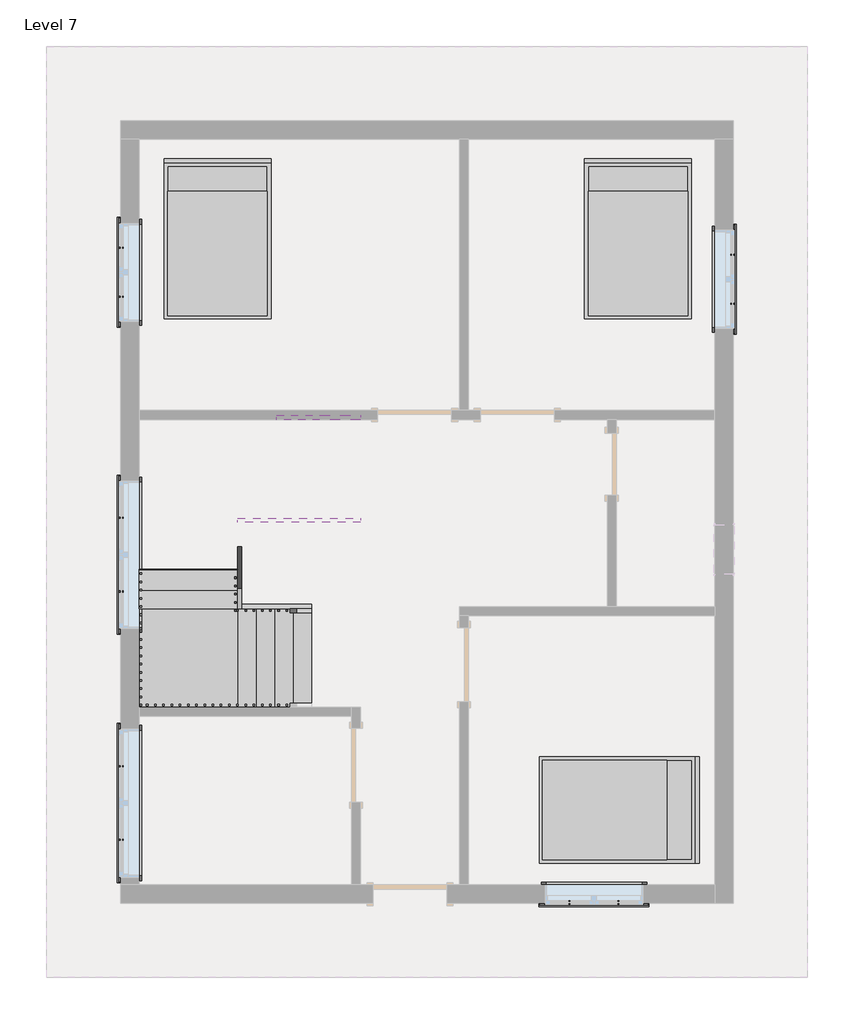
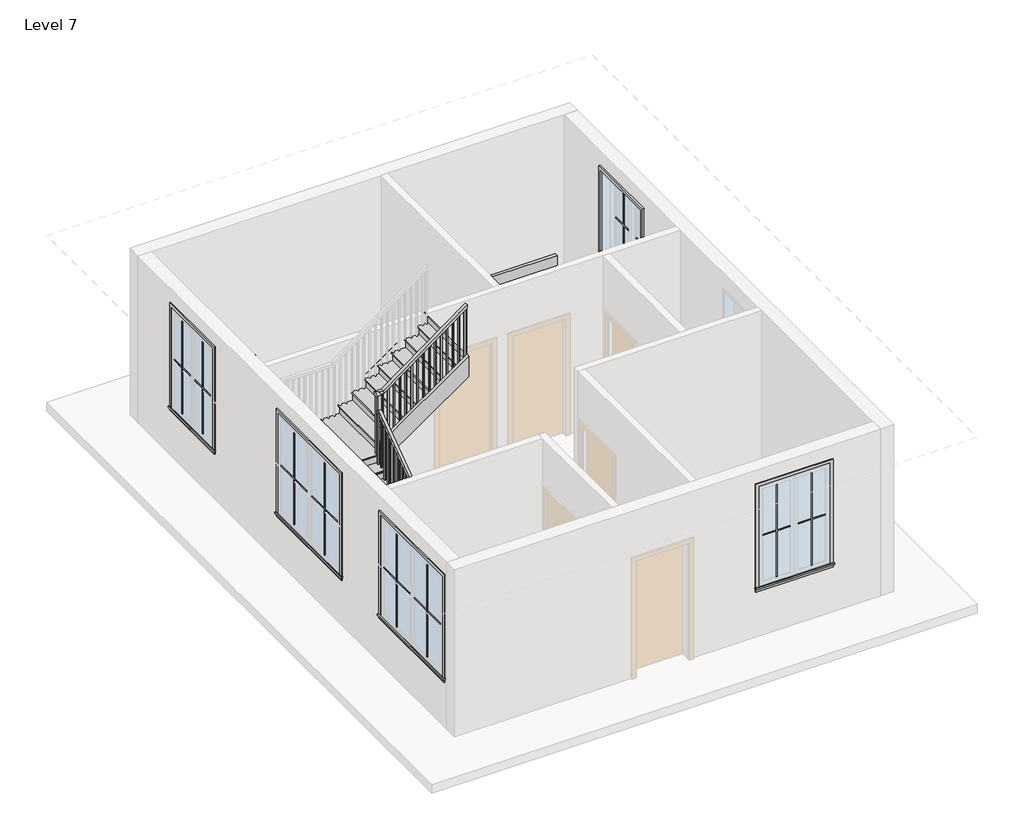
# One storey, part 3 of 3: 20 proxies, 5 members, 3 furniture elements, 1 railing, 1 stair flight.
"""IFC4 building model written with IfcOpenShell, lengths in millimetres."""

from ifc_helpers import new_model, si_unit, frame, origin, place, context, project, spatial, polyline, outline, extrude, faceted_brep, transform, mapped, element, save
from components import muntin_pattern_2x2_muntin_pattern_2x2_0a037076, muntin_pattern_2x2_muntin_pattern_2x2_e6f69628, muntin_pattern_2x2_muntin_pattern_2x2_2b4d9f72, muntin_pattern_2x2_muntin_pattern_2x2_ef995ed3, trim_window_exterior_flat_with_sill_b601e94a, trim_window_exterior_flat_with_sill_b7e4d11c, trim_window_interior_flat_picture_frame_bfefb25c, trim_window_interior_flat_picture_frame_936b8d2a, bed_17739_bed_17739_15c61121, stair_flight_f77ae209

model = new_model("IFC4")

# Units and contexts
model_context = context("Model", 3, world=origin())
ifc_project = project(units=[si_unit("LENGTHUNIT", "METRE", prefix="MILLI")], contexts=[model_context])

# Site, building, storey
site = spatial("IfcSite", under=ifc_project)
building = spatial("IfcBuilding", under=site)
storey = spatial("IfcBuildingStorey", under=building, Name="Level 7", Elevation=19050.0)

# Proxies
placement = place(None, origin())
muntin_pattern_2x2_muntin_pattern_2x2_shape = muntin_pattern_2x2_muntin_pattern_2x2_0a037076(model_context)
element("IfcBuildingElementProxy", 1, Name="Muntin Pattern_2x2 : Muntin Pattern_2x2", ObjectType="Muntin Pattern_2x2 : Muntin Pattern_2x2", at=placement, inside=storey, context=model_context, shape_type="MappedRepresentation", body=[
    mapped(muntin_pattern_2x2_muntin_pattern_2x2_shape, transform((-5035.7855391, -4380.9248761, 20034.25), x_axis=(0.0, 1.0, 0.0), y_axis=(-1.0, 0.0, 0.0), z_axis=(0.0, 0.0, 1.0))),
])
element("IfcBuildingElementProxy", 2, Name="Muntin Pattern_2x2 : Muntin Pattern_2x2", ObjectType="Muntin Pattern_2x2 : Muntin Pattern_2x2", at=placement, inside=storey, context=model_context, shape_type="MappedRepresentation", body=[
    mapped(muntin_pattern_2x2_muntin_pattern_2x2_shape, transform((-5035.7855391, -1310.6998761, 20034.25), x_axis=(0.0, 1.0, 0.0), y_axis=(-1.0, 0.0, 0.0), z_axis=(0.0, 0.0, 1.0))),
])
muntin_pattern_2x2_muntin_pattern_2x2_2_shape = muntin_pattern_2x2_muntin_pattern_2x2_e6f69628(model_context)
element("IfcBuildingElementProxy", 3, Name="Muntin Pattern_2x2 : Muntin Pattern_2x2", ObjectType="Muntin Pattern_2x2 : Muntin Pattern_2x2", at=placement, inside=storey, context=model_context, shape_type="MappedRepresentation", body=[
    mapped(muntin_pattern_2x2_muntin_pattern_2x2_2_shape, transform((-5035.7855391, -3469.6998761, 20034.25), x_axis=(0.0, -1.0, 0.0), y_axis=(1.0, 0.0, 0.0), z_axis=(0.0, 0.0, 1.0))),
])
element("IfcBuildingElementProxy", 4, Name="Muntin Pattern_2x2 : Muntin Pattern_2x2", ObjectType="Muntin Pattern_2x2 : Muntin Pattern_2x2", at=placement, inside=storey, context=model_context, shape_type="MappedRepresentation", body=[
    mapped(muntin_pattern_2x2_muntin_pattern_2x2_2_shape, transform((-5035.7855391, -399.4748761, 20034.25), x_axis=(0.0, -1.0, 0.0), y_axis=(1.0, 0.0, 0.0), z_axis=(0.0, 0.0, 1.0))),
])
muntin_pattern_2x2_muntin_pattern_2x2_3_shape = muntin_pattern_2x2_muntin_pattern_2x2_2b4d9f72(model_context)
element("IfcBuildingElementProxy", 5, Name="Muntin Pattern_2x2 : Muntin Pattern_2x2", ObjectType="Muntin Pattern_2x2 : Muntin Pattern_2x2", at=placement, inside=storey, context=model_context, shape_type="MappedRepresentation", body=[
    mapped(muntin_pattern_2x2_muntin_pattern_2x2_3_shape, transform((1115.7769609, -5157.2123761, 20034.25), x_axis=(-1.0, 0.0, 0.0), y_axis=(0.0, -1.0, 0.0), z_axis=(0.0, 0.0, 1.0))),
])
element("IfcBuildingElementProxy", 6, Name="Muntin Pattern_2x2 : Muntin Pattern_2x2", ObjectType="Muntin Pattern_2x2 : Muntin Pattern_2x2", at=placement, inside=storey, context=model_context, shape_type="MappedRepresentation", body=[
    mapped(muntin_pattern_2x2_muntin_pattern_2x2_3_shape, transform((2527.0644609, 2851.7251239, 20034.25), x_axis=(0.0, -1.0, 0.0), y_axis=(1.0, 0.0, 0.0), z_axis=(0.0, 0.0, 1.0))),
])
element("IfcBuildingElementProxy", 7, Name="Muntin Pattern_2x2 : Muntin Pattern_2x2", ObjectType="Muntin Pattern_2x2 : Muntin Pattern_2x2", at=placement, inside=storey, context=model_context, shape_type="MappedRepresentation", body=[
    mapped(muntin_pattern_2x2_muntin_pattern_2x2_3_shape, transform((-5035.7855391, 2331.0251239, 20034.25), x_axis=(0.0, 1.0, 0.0), y_axis=(-1.0, 0.0, 0.0), z_axis=(0.0, 0.0, 1.0))),
])
muntin_pattern_2x2_muntin_pattern_2x2_4_shape = muntin_pattern_2x2_muntin_pattern_2x2_ef995ed3(model_context)
element("IfcBuildingElementProxy", 8, Name="Muntin Pattern_2x2 : Muntin Pattern_2x2", ObjectType="Muntin Pattern_2x2 : Muntin Pattern_2x2", at=placement, inside=storey, context=model_context, shape_type="MappedRepresentation", body=[
    mapped(muntin_pattern_2x2_muntin_pattern_2x2_4_shape, transform((509.3519609, -5157.2123761, 20034.25), x_axis=(1.0, 0.0, 0.0), y_axis=(0.0, 1.0, 0.0), z_axis=(0.0, 0.0, 1.0))),
])
element("IfcBuildingElementProxy", 9, Name="Muntin Pattern_2x2 : Muntin Pattern_2x2", ObjectType="Muntin Pattern_2x2 : Muntin Pattern_2x2", at=placement, inside=storey, context=model_context, shape_type="MappedRepresentation", body=[
    mapped(muntin_pattern_2x2_muntin_pattern_2x2_4_shape, transform((2527.0644609, 2245.3001239, 20034.25), x_axis=(0.0, 1.0, 0.0), y_axis=(-1.0, 0.0, 0.0), z_axis=(0.0, 0.0, 1.0))),
])
element("IfcBuildingElementProxy", 10, Name="Muntin Pattern_2x2 : Muntin Pattern_2x2", ObjectType="Muntin Pattern_2x2 : Muntin Pattern_2x2", at=placement, inside=storey, context=model_context, shape_type="MappedRepresentation", body=[
    mapped(muntin_pattern_2x2_muntin_pattern_2x2_4_shape, transform((-5035.7855391, 2937.4501239, 20034.25), x_axis=(0.0, -1.0, 0.0), y_axis=(1.0, 0.0, 0.0), z_axis=(0.0, 0.0, 1.0))),
])
trim_window_exterior_flat_with_sill_shape = trim_window_exterior_flat_with_sill_b601e94a(model_context)
element("IfcBuildingElementProxy", 11, Name="Trim-Window-Exterior-Flat : with Sill", ObjectType="Trim-Window-Exterior-Flat : with Sill", at=placement, inside=storey, context=model_context, shape_type="MappedRepresentation", body=[
    mapped(trim_window_exterior_flat_with_sill_shape, transform((-5045.3105391, -3925.3123761, 21793.2), x_axis=(0.0, -1.0, 0.0), y_axis=(0.0, 0.0, 1.0), z_axis=(-1.0, 0.0, 0.0))),
])
element("IfcBuildingElementProxy", 12, Name="Trim-Window-Exterior-Flat : with Sill", ObjectType="Trim-Window-Exterior-Flat : with Sill", at=placement, inside=storey, context=model_context, shape_type="MappedRepresentation", body=[
    mapped(trim_window_exterior_flat_with_sill_shape, transform((-5045.3105391, -855.0873761, 21793.2), x_axis=(0.0, -1.0, 0.0), y_axis=(0.0, 0.0, 1.0), z_axis=(-1.0, 0.0, 0.0))),
])
trim_window_exterior_flat_with_sill_2_shape = trim_window_exterior_flat_with_sill_b7e4d11c(model_context)
element("IfcBuildingElementProxy", 13, Name="Trim-Window-Exterior-Flat : with Sill", ObjectType="Trim-Window-Exterior-Flat : with Sill", at=placement, inside=storey, context=model_context, shape_type="MappedRepresentation", body=[
    mapped(trim_window_exterior_flat_with_sill_2_shape, transform((812.5644609, -5166.7373761, 21793.2), x_axis=(1.0, 0.0, 0.0), y_axis=(0.0, 0.0, 1.0), z_axis=(0.0, -1.0, 0.0))),
])
element("IfcBuildingElementProxy", 14, Name="Trim-Window-Exterior-Flat : with Sill", ObjectType="Trim-Window-Exterior-Flat : with Sill", at=placement, inside=storey, context=model_context, shape_type="MappedRepresentation", body=[
    mapped(trim_window_exterior_flat_with_sill_2_shape, transform((2536.5894609, 2548.5126239, 21793.2), x_axis=(0.0, 1.0, 0.0), y_axis=(0.0, 0.0, 1.0), z_axis=(1.0, 0.0, 0.0))),
])
element("IfcBuildingElementProxy", 15, Name="Trim-Window-Exterior-Flat : with Sill", ObjectType="Trim-Window-Exterior-Flat : with Sill", at=placement, inside=storey, context=model_context, shape_type="MappedRepresentation", body=[
    mapped(trim_window_exterior_flat_with_sill_2_shape, transform((-5045.3105391, 2634.2376239, 21793.2), x_axis=(0.0, -1.0, 0.0), y_axis=(0.0, 0.0, 1.0), z_axis=(-1.0, 0.0, 0.0))),
])
trim_window_interior_flat_picture_frame_shape = trim_window_interior_flat_picture_frame_bfefb25c(model_context)
element("IfcBuildingElementProxy", 16, Name="Trim-Window-Interior-Flat : Picture Frame", ObjectType="Trim-Window-Interior-Flat : Picture Frame", at=placement, inside=storey, context=model_context, shape_type="MappedRepresentation", body=[
    mapped(trim_window_interior_flat_picture_frame_shape, transform((-4816.7105391, -3925.3123761, 21793.2), x_axis=(0.0, 1.0, 0.0), y_axis=(0.0, 0.0, 1.0), z_axis=(1.0, 0.0, 0.0))),
])
element("IfcBuildingElementProxy", 17, Name="Trim-Window-Interior-Flat : Picture Frame", ObjectType="Trim-Window-Interior-Flat : Picture Frame", at=placement, inside=storey, context=model_context, shape_type="MappedRepresentation", body=[
    mapped(trim_window_interior_flat_picture_frame_shape, transform((-4816.7105391, -855.0873761, 21793.2), x_axis=(0.0, 1.0, 0.0), y_axis=(0.0, 0.0, 1.0), z_axis=(1.0, 0.0, 0.0))),
])
trim_window_interior_flat_picture_frame_2_shape = trim_window_interior_flat_picture_frame_936b8d2a(model_context)
element("IfcBuildingElementProxy", 18, Name="Trim-Window-Interior-Flat : Picture Frame", ObjectType="Trim-Window-Interior-Flat : Picture Frame", at=placement, inside=storey, context=model_context, shape_type="MappedRepresentation", body=[
    mapped(trim_window_interior_flat_picture_frame_2_shape, transform((812.5644609, -4938.1373761, 21793.2), x_axis=(-1.0, 0.0, 0.0), y_axis=(0.0, 0.0, 1.0), z_axis=(0.0, 1.0, 0.0))),
])
element("IfcBuildingElementProxy", 19, Name="Trim-Window-Interior-Flat : Picture Frame", ObjectType="Trim-Window-Interior-Flat : Picture Frame", at=placement, inside=storey, context=model_context, shape_type="MappedRepresentation", body=[
    mapped(trim_window_interior_flat_picture_frame_2_shape, transform((2307.9894609, 2548.5126239, 21793.2), x_axis=(0.0, -1.0, 0.0), y_axis=(0.0, 0.0, 1.0), z_axis=(-1.0, 0.0, 0.0))),
])
element("IfcBuildingElementProxy", 20, Name="Trim-Window-Interior-Flat : Picture Frame", ObjectType="Trim-Window-Interior-Flat : Picture Frame", at=placement, inside=storey, context=model_context, shape_type="MappedRepresentation", body=[
    mapped(trim_window_interior_flat_picture_frame_2_shape, transform((-4816.7105391, 2634.2376239, 21793.2), x_axis=(0.0, 1.0, 0.0), y_axis=(0.0, 0.0, 1.0), z_axis=(1.0, 0.0, 0.0))),
])

# Furniture
bed_17739_bed_17739_shape = bed_17739_bed_17739_15c61121(model_context)
element("IfcFurniture", 21, ObjectType="Bed_17739 : Bed_17739", at=placement, inside=storey, context=model_context, shape_type="MappedRepresentation", body=[
    mapped(bed_17739_bed_17739_shape, transform((-3845.1605391, 3024.7626239, 19050.0), x_axis=(1.0, 0.0, 0.0), y_axis=(0.0, 1.0, 0.0), z_axis=(0.0, 0.0, 1.0))),
])
element("IfcFurniture", 22, ObjectType="Bed_17739 : Bed_17739", at=placement, inside=storey, context=model_context, shape_type="MappedRepresentation", body=[
    mapped(bed_17739_bed_17739_shape, transform((1355.4894609, 3024.7626239, 19050.0), x_axis=(1.0, 0.0, 0.0), y_axis=(0.0, 1.0, 0.0), z_axis=(0.0, 0.0, 1.0))),
])
element("IfcFurniture", 23, ObjectType="Bed_17739 : Bed_17739", at=placement, inside=storey, context=model_context, shape_type="MappedRepresentation", body=[
    mapped(bed_17739_bed_17739_shape, transform((1101.4894609, -4011.0373761, 19050.0), x_axis=(0.0, -1.0, 0.0), y_axis=(1.0, 0.0, 0.0), z_axis=(0.0, 0.0, 1.0))),
])

# Members
element("IfcMember", 24, ObjectType="Stringer - 2\" Width", at=placement, inside=storey, context=model_context, shape_type="SweptSolid", body=[
    extrude(outline(polyline([(19050.0, -2683.1105391), (19200.5087903, -2683.1105391), (19200.5087903, -3112.2707489), (19050.0, -2897.7957228), (19050.0, -2683.1105391)])), frame((0.0, -2791.8373761, 0.0), z_axis=(0.0, 1.0, 0.0), x_axis=(0.0, 0.0, 1.0)), (0.0, 0.0, 1.0), 50.8),
])
element("IfcMember", 25, ObjectType="Stringer - 2\" Width", at=placement, inside=storey, context=model_context, shape_type="SweptSolid", body=[
    extrude(outline(polyline([(21377.4856495, -2580.7583047), (21733.4489938, -2073.5105391), (22105.8117181, -2073.5105391), (21377.4856495, -3111.3751869), (21377.4856495, -2580.7583047)])), frame((0.0, 814.9626239, 0.0), z_axis=(0.0, 1.0, 0.0), x_axis=(0.0, 0.0, 1.0)), (0.0, 0.0, 1.0), 50.8),
])
element("IfcMember", 26, ObjectType="Stringer - 2\" Width", at=placement, inside=storey, context=model_context, shape_type="SweptSolid", body=[
    extrude(outline(polyline([(19050.0, -2683.1105391), (19271.706455, -2683.1105391), (19877.7415427, -3546.7105391), (19505.3788184, -3546.7105391), (19050.0, -2897.7957228), (19050.0, -2683.1105391)])), frame((0.0, -1521.8373761, 0.0), z_axis=(0.0, 1.0, 0.0), x_axis=(0.0, 0.0, 1.0)), (0.0, 0.0, 1.0), 50.8),
])
element("IfcMember", 27, ObjectType="Stringer - 2\" Width", at=placement, inside=storey, context=model_context, shape_type="SweptSolid", body=[
    extrude(outline(polyline([(-1521.8373761, 19700.3564629), (-1521.8373761, 20075.5327137), (-455.0373761, 20841.1786467), (-455.0373761, 20466.0023959), (-1521.8373761, 19700.3564629)])), frame((-3597.5105391, 0.0, 0.0), z_axis=(1.0, 0.0, 0.0), x_axis=(0.0, 1.0, 0.0)), (0.0, 0.0, 1.0), 50.8),
])
element("IfcMember", 28, ObjectType="Stringer - 2\" Width", at=placement, inside=storey, context=model_context, shape_type="SweptSolid", body=[
    extrude(outline(polyline([(21036.3380339, -3597.5105391), (20663.9753096, -3597.5105391), (21733.4489938, -2073.5105391), (22105.8117181, -2073.5105391), (21036.3380339, -3597.5105391)])), frame((0.0, -455.0373761, 0.0), z_axis=(0.0, 1.0, 0.0), x_axis=(0.0, 0.0, 1.0)), (0.0, 0.0, 1.0), 50.8),
])

# Railing
element("IfcRailing", 29, ObjectType="Handrail - Rectangular", at=placement, inside=storey, context=model_context, shape_type="SolidModel", body=[
    faceted_brep([(-2683.1105391, -1572.6373761, 20124.8210526), (-2683.1105391, -1572.6373761, 20062.7605986), (-2683.1105391, -1521.8373761, 20062.7605986), (-2683.1105391, -1521.8373761, 20124.8210526), (-3521.3105391, -1572.6373761, 20713.0315789), (-3572.1105391, -1572.6373761, 20686.6202477), (-3572.1105391, -1521.8373761, 20686.6202477), (-3521.3105391, -1521.8373761, 20713.0315789), (-3521.3105391, -1572.6373761, 20981.615311), (-3572.1105391, -1572.6373761, 20930.815311), (-3572.1105391, -1521.8373761, 20930.815311), (-3521.3105391, -1521.8373761, 20981.615311), (-3648.3105391, -1572.6373761, 20981.615311), (-3648.3105391, -1572.6373761, 20930.815311), (-3597.5105391, -1521.8373761, 20930.815311), (-3597.5105391, -1521.8373761, 20981.615311), (-3648.3105391, -1445.6373761, 20981.615311), (-3648.3105391, -1429.2944467, 20930.815311), (-3597.5105391, -1429.2944467, 20930.815311), (-3597.5105391, -1445.6373761, 20981.615311), (-3648.3105391, -480.4373761, 21674.3425837), (-3648.3105391, -429.6373761, 21648.2725387), (-3597.5105391, -429.6373761, 21648.2725387), (-3597.5105391, -480.4373761, 21674.3425837), (-3648.3105391, -480.4373761, 21945.6), (-3648.3105391, -429.6373761, 21894.8), (-3597.5105391, -429.6373761, 21894.8), (-3597.5105391, -480.4373761, 21945.6), (-3648.3105391, -353.4373761, 21945.6), (-3648.3105391, -353.4373761, 21894.8), (-3597.5105391, -404.2373761, 21894.8), (-3597.5105391, -404.2373761, 21945.6), (-3521.3105391, -353.4373761, 21945.6), (-3504.6160355, -353.4373761, 21894.8), (-3504.6160355, -404.2373761, 21894.8), (-3521.3105391, -404.2373761, 21945.6), (-2073.5105391, -353.4373761, 23012.4), (-2073.5105391, -404.2373761, 23012.4), (-2073.5105391, -404.2373761, 22949.2987868), (-2073.5105391, -353.4373761, 22949.2987868)], [[[0, 1, 2, 3]], [[1, 0, 4, 5]], [[2, 1, 5, 6]], [[3, 2, 6, 7]], [[0, 3, 7, 4]], [[5, 4, 8, 9]], [[6, 5, 9, 10]], [[7, 6, 10, 11]], [[4, 7, 11, 8]], [[9, 8, 12, 13]], [[10, 9, 13, 14]], [[11, 10, 14, 15]], [[8, 11, 15, 12]], [[13, 12, 16, 17]], [[14, 13, 17, 18]], [[15, 14, 18, 19]], [[12, 15, 19, 16]], [[17, 16, 20, 21]], [[18, 17, 21, 22]], [[19, 18, 22, 23]], [[16, 19, 23, 20]], [[21, 20, 24, 25]], [[22, 21, 25, 26]], [[23, 22, 26, 27]], [[20, 23, 27, 24]], [[25, 24, 28, 29]], [[26, 25, 29, 30]], [[27, 26, 30, 31]], [[24, 27, 31, 28]], [[29, 28, 32, 33]], [[30, 29, 33, 34]], [[31, 30, 34, 35]], [[28, 31, 35, 32]], [[36, 37, 38, 39]], [[33, 32, 36, 39]], [[34, 33, 39, 38]], [[35, 34, 38, 37]], [[32, 35, 37, 36]]]),
    extrude(outline(polyline([(22937.6014184, -2089.3855391), (22923.5645763, -2108.4355391), (21937.5789474, -2108.4355391), (21937.5789474, -2089.3855391), (22937.6014184, -2089.3855391)])), frame((0.0, -388.3623761, 0.0), z_axis=(0.0, 1.0, 0.0), x_axis=(0.0, 0.0, 1.0)), (0.0, 0.0, 1.0), 19.05),
    extrude(outline(polyline([(22862.7382605, -2190.9855391), (22848.7014184, -2210.0355391), (21937.5789474, -2210.0355391), (21937.5789474, -2190.9855391), (22862.7382605, -2190.9855391)])), frame((0.0, -388.3623761, 0.0), z_axis=(0.0, 1.0, 0.0), x_axis=(0.0, 0.0, 1.0)), (0.0, 0.0, 1.0), 19.05),
    extrude(outline(polyline([(22787.8751026, -2292.5855391), (22773.8382605, -2311.6355391), (21777.1578947, -2311.6355391), (21777.1578947, -2292.5855391), (22787.8751026, -2292.5855391)])), frame((0.0, -388.3623761, 0.0), z_axis=(0.0, 1.0, 0.0), x_axis=(0.0, 0.0, 1.0)), (0.0, 0.0, 1.0), 19.05),
    extrude(outline(polyline([(22713.0119447, -2394.1855391), (22698.9751026, -2413.2355391), (21777.1578947, -2413.2355391), (21777.1578947, -2394.1855391), (22713.0119447, -2394.1855391)])), frame((0.0, -388.3623761, 0.0), z_axis=(0.0, 1.0, 0.0), x_axis=(0.0, 0.0, 1.0)), (0.0, 0.0, 1.0), 19.05),
    extrude(outline(polyline([(22638.1487868, -2495.7855391), (22624.1119447, -2514.8355391), (21616.7368421, -2514.8355391), (21616.7368421, -2495.7855391), (22638.1487868, -2495.7855391)])), frame((0.0, -388.3623761, 0.0), z_axis=(0.0, 1.0, 0.0), x_axis=(0.0, 0.0, 1.0)), (0.0, 0.0, 1.0), 19.05),
    extrude(outline(polyline([(22563.2856289, -2597.3855391), (22549.2487868, -2616.4355391), (21616.7368421, -2616.4355391), (21616.7368421, -2597.3855391), (22563.2856289, -2597.3855391)])), frame((0.0, -388.3623761, 0.0), z_axis=(0.0, 1.0, 0.0), x_axis=(0.0, 0.0, 1.0)), (0.0, 0.0, 1.0), 19.05),
    extrude(outline(polyline([(22488.422471, -2698.9855391), (22474.3856289, -2718.0355391), (21456.3157895, -2718.0355391), (21456.3157895, -2698.9855391), (22488.422471, -2698.9855391)])), frame((0.0, -388.3623761, 0.0), z_axis=(0.0, 1.0, 0.0), x_axis=(0.0, 0.0, 1.0)), (0.0, 0.0, 1.0), 19.05),
    extrude(outline(polyline([(22413.5593132, -2800.5855391), (22399.522471, -2819.6355391), (21456.3157895, -2819.6355391), (21456.3157895, -2800.5855391), (22413.5593132, -2800.5855391)])), frame((0.0, -388.3623761, 0.0), z_axis=(0.0, 1.0, 0.0), x_axis=(0.0, 0.0, 1.0)), (0.0, 0.0, 1.0), 19.05),
    extrude(outline(polyline([(22338.6961553, -2902.1855391), (22324.6593132, -2921.2355391), (21456.3157895, -2921.2355391), (21456.3157895, -2902.1855391), (22338.6961553, -2902.1855391)])), frame((0.0, -388.3623761, 0.0), z_axis=(0.0, 1.0, 0.0), x_axis=(0.0, 0.0, 1.0)), (0.0, 0.0, 1.0), 19.05),
    extrude(outline(polyline([(22263.8329974, -3003.7855391), (22249.7961553, -3022.8355391), (21295.8947368, -3022.8355391), (21295.8947368, -3003.7855391), (22263.8329974, -3003.7855391)])), frame((0.0, -388.3623761, 0.0), z_axis=(0.0, 1.0, 0.0), x_axis=(0.0, 0.0, 1.0)), (0.0, 0.0, 1.0), 19.05),
    extrude(outline(polyline([(22188.9698395, -3105.3855391), (22174.9329974, -3124.4355391), (21295.8947368, -3124.4355391), (21295.8947368, -3105.3855391), (22188.9698395, -3105.3855391)])), frame((0.0, -388.3623761, 0.0), z_axis=(0.0, 1.0, 0.0), x_axis=(0.0, 0.0, 1.0)), (0.0, 0.0, 1.0), 19.05),
    extrude(outline(polyline([(22114.1066816, -3206.9855391), (22100.0698395, -3226.0355391), (21135.4736842, -3226.0355391), (21135.4736842, -3206.9855391), (22114.1066816, -3206.9855391)])), frame((0.0, -388.3623761, 0.0), z_axis=(0.0, 1.0, 0.0), x_axis=(0.0, 0.0, 1.0)), (0.0, 0.0, 1.0), 19.05),
    extrude(outline(polyline([(22039.2435237, -3308.5855391), (22025.2066816, -3327.6355391), (21135.4736842, -3327.6355391), (21135.4736842, -3308.5855391), (22039.2435237, -3308.5855391)])), frame((0.0, -388.3623761, 0.0), z_axis=(0.0, 1.0, 0.0), x_axis=(0.0, 0.0, 1.0)), (0.0, 0.0, 1.0), 19.05),
    extrude(outline(polyline([(21964.3803658, -3410.1855391), (21950.3435237, -3429.2355391), (20975.0526316, -3429.2355391), (20975.0526316, -3410.1855391), (21964.3803658, -3410.1855391)])), frame((0.0, -388.3623761, 0.0), z_axis=(0.0, 1.0, 0.0), x_axis=(0.0, 0.0, 1.0)), (0.0, 0.0, 1.0), 19.05),
    extrude(outline(polyline([(21889.5172079, -3511.7855391), (21875.4803658, -3530.8355391), (20975.0526316, -3530.8355391), (20975.0526316, -3511.7855391), (21889.5172079, -3511.7855391)])), frame((0.0, -388.3623761, 0.0), z_axis=(0.0, 1.0, 0.0), x_axis=(0.0, 0.0, 1.0)), (0.0, 0.0, 1.0), 19.05),
    extrude(outline(polyline([(-3613.3855391, -439.1623761), (-3632.4355391, -439.1623761), (-3632.4355391, -420.1123761), (-3613.3855391, -420.1123761), (-3613.3855391, -439.1623761)])), frame((0.0, 0.0, 20654.2105263), z_axis=(0.0, 0.0, 1.0), x_axis=(1.0, 0.0, 0.0)), (0.0, 0.0, 1.0), 1240.5894737),
    extrude(outline(polyline([(-540.7623761, 21568.5177541), (-521.7123761, 21582.1900029), (-521.7123761, 20654.2105263), (-540.7623761, 20654.2105263), (-540.7623761, 21568.5177541)])), frame((-3632.4355391, 0.0, 0.0), z_axis=(1.0, 0.0, 0.0), x_axis=(0.0, 1.0, 0.0)), (0.0, 0.0, 1.0), 19.05),
    extrude(outline(polyline([(-642.3623761, 21495.5990938), (-623.3123761, 21509.2713426), (-623.3123761, 20493.7894737), (-642.3623761, 20493.7894737), (-642.3623761, 21495.5990938)])), frame((-3632.4355391, 0.0, 0.0), z_axis=(1.0, 0.0, 0.0), x_axis=(0.0, 1.0, 0.0)), (0.0, 0.0, 1.0), 19.05),
    extrude(outline(polyline([(-743.9623761, 21422.6804335), (-724.9123761, 21436.3526823), (-724.9123761, 20493.7894737), (-743.9623761, 20493.7894737), (-743.9623761, 21422.6804335)])), frame((-3632.4355391, 0.0, 0.0), z_axis=(1.0, 0.0, 0.0), x_axis=(0.0, 1.0, 0.0)), (0.0, 0.0, 1.0), 19.05),
    extrude(outline(polyline([(-845.5623761, 21349.7617732), (-826.5123761, 21363.434022), (-826.5123761, 20493.7894737), (-845.5623761, 20493.7894737), (-845.5623761, 21349.7617732)])), frame((-3632.4355391, 0.0, 0.0), z_axis=(1.0, 0.0, 0.0), x_axis=(0.0, 1.0, 0.0)), (0.0, 0.0, 1.0), 19.05),
    extrude(outline(polyline([(-947.1623761, 21276.8431129), (-928.1123761, 21290.5153617), (-928.1123761, 20333.3684211), (-947.1623761, 20333.3684211), (-947.1623761, 21276.8431129)])), frame((-3632.4355391, 0.0, 0.0), z_axis=(1.0, 0.0, 0.0), x_axis=(0.0, 1.0, 0.0)), (0.0, 0.0, 1.0), 19.05),
    extrude(outline(polyline([(-1048.7623761, 21203.9244526), (-1029.7123761, 21217.5967014), (-1029.7123761, 20333.3684211), (-1048.7623761, 20333.3684211), (-1048.7623761, 21203.9244526)])), frame((-3632.4355391, 0.0, 0.0), z_axis=(1.0, 0.0, 0.0), x_axis=(0.0, 1.0, 0.0)), (0.0, 0.0, 1.0), 19.05),
    extrude(outline(polyline([(-1150.3623761, 21131.0057923), (-1131.3123761, 21144.6780411), (-1131.3123761, 20172.9473684), (-1150.3623761, 20172.9473684), (-1150.3623761, 21131.0057923)])), frame((-3632.4355391, 0.0, 0.0), z_axis=(1.0, 0.0, 0.0), x_axis=(0.0, 1.0, 0.0)), (0.0, 0.0, 1.0), 19.05),
    extrude(outline(polyline([(-1251.9623761, 21058.087132), (-1232.9123761, 21071.7593808), (-1232.9123761, 20172.9473684), (-1251.9623761, 20172.9473684), (-1251.9623761, 21058.087132)])), frame((-3632.4355391, 0.0, 0.0), z_axis=(1.0, 0.0, 0.0), x_axis=(0.0, 1.0, 0.0)), (0.0, 0.0, 1.0), 19.05),
    extrude(outline(polyline([(-1353.5623761, 20985.1684718), (-1334.5123761, 20998.8407206), (-1334.5123761, 20012.5263158), (-1353.5623761, 20012.5263158), (-1353.5623761, 20985.1684718)])), frame((-3632.4355391, 0.0, 0.0), z_axis=(1.0, 0.0, 0.0), x_axis=(0.0, 1.0, 0.0)), (0.0, 0.0, 1.0), 19.05),
    extrude(outline(polyline([(-1455.1623761, 20912.2498115), (-1436.1123761, 20925.9220603), (-1436.1123761, 20012.5263158), (-1455.1623761, 20012.5263158), (-1455.1623761, 20912.2498115)])), frame((-3632.4355391, 0.0, 0.0), z_axis=(1.0, 0.0, 0.0), x_axis=(0.0, 1.0, 0.0)), (0.0, 0.0, 1.0), 19.05),
    extrude(outline(polyline([(-3587.9855391, -1537.7123761), (-3587.9855391, -1556.7623761), (-3607.0355391, -1556.7623761), (-3607.0355391, -1537.7123761), (-3587.9855391, -1537.7123761)])), frame((0.0, 0.0, 19852.1052632), z_axis=(0.0, 0.0, 1.0), x_axis=(1.0, 0.0, 0.0)), (0.0, 0.0, 1.0), 1078.7100478),
    extrude(outline(polyline([(20626.462353, -3486.3855391), (20639.830774, -3505.4355391), (19691.6842105, -3505.4355391), (19691.6842105, -3486.3855391), (20626.462353, -3486.3855391)])), frame((0.0, -1556.7623761, 0.0), z_axis=(0.0, 1.0, 0.0), x_axis=(0.0, 0.0, 1.0)), (0.0, 0.0, 1.0), 19.05),
    extrude(outline(polyline([(20555.1641074, -3384.7855391), (20568.5325284, -3403.8355391), (19691.6842105, -3403.8355391), (19691.6842105, -3384.7855391), (20555.1641074, -3384.7855391)])), frame((0.0, -1556.7623761, 0.0), z_axis=(0.0, 1.0, 0.0), x_axis=(0.0, 0.0, 1.0)), (0.0, 0.0, 1.0), 19.05),
    extrude(outline(polyline([(20483.8658617, -3283.1855391), (20497.2342828, -3302.2355391), (19531.2631579, -3302.2355391), (19531.2631579, -3283.1855391), (20483.8658617, -3283.1855391)])), frame((0.0, -1556.7623761, 0.0), z_axis=(0.0, 1.0, 0.0), x_axis=(0.0, 0.0, 1.0)), (0.0, 0.0, 1.0), 19.05),
    extrude(outline(polyline([(20412.5676161, -3181.5855391), (20425.9360372, -3200.6355391), (19531.2631579, -3200.6355391), (19531.2631579, -3181.5855391), (20412.5676161, -3181.5855391)])), frame((0.0, -1556.7623761, 0.0), z_axis=(0.0, 1.0, 0.0), x_axis=(0.0, 0.0, 1.0)), (0.0, 0.0, 1.0), 19.05),
    extrude(outline(polyline([(20341.2693705, -3079.9855391), (20354.6377916, -3099.0355391), (19370.8421053, -3099.0355391), (19370.8421053, -3079.9855391), (20341.2693705, -3079.9855391)])), frame((0.0, -1556.7623761, 0.0), z_axis=(0.0, 1.0, 0.0), x_axis=(0.0, 0.0, 1.0)), (0.0, 0.0, 1.0), 19.05),
    extrude(outline(polyline([(20269.9711249, -2978.3855391), (20283.3395459, -2997.4355391), (19370.8421053, -2997.4355391), (19370.8421053, -2978.3855391), (20269.9711249, -2978.3855391)])), frame((0.0, -1556.7623761, 0.0), z_axis=(0.0, 1.0, 0.0), x_axis=(0.0, 0.0, 1.0)), (0.0, 0.0, 1.0), 19.05),
    extrude(outline(polyline([(20198.6728793, -2876.7855391), (20212.0413003, -2895.8355391), (19210.4210526, -2895.8355391), (19210.4210526, -2876.7855391), (20198.6728793, -2876.7855391)])), frame((0.0, -1556.7623761, 0.0), z_axis=(0.0, 1.0, 0.0), x_axis=(0.0, 0.0, 1.0)), (0.0, 0.0, 1.0), 19.05),
    extrude(outline(polyline([(20127.3746337, -2775.1855391), (20140.7430547, -2794.2355391), (19210.4210526, -2794.2355391), (19210.4210526, -2775.1855391), (20127.3746337, -2775.1855391)])), frame((0.0, -1556.7623761, 0.0), z_axis=(0.0, 1.0, 0.0), x_axis=(0.0, 0.0, 1.0)), (0.0, 0.0, 1.0), 19.05),
    extrude(outline(polyline([(-3613.3855391, -388.3623761), (-3632.4355391, -388.3623761), (-3632.4355391, -369.3123761), (-3613.3855391, -369.3123761), (-3613.3855391, -388.3623761)])), frame((0.0, 0.0, 20814.6315789), z_axis=(0.0, 0.0, 1.0), x_axis=(1.0, 0.0, 0.0)), (0.0, 0.0, 1.0), 1080.1684211),
    extrude(outline(polyline([(-3613.3855391, -1537.7123761), (-3613.3855391, -1556.7623761), (-3632.4355391, -1556.7623761), (-3632.4355391, -1537.7123761), (-3613.3855391, -1537.7123761)])), frame((0.0, 0.0, 19852.1052632), z_axis=(0.0, 0.0, 1.0), x_axis=(1.0, 0.0, 0.0)), (0.0, 0.0, 1.0), 1078.7100478),
    extrude(outline(polyline([(22949.2987868, -2073.5105391), (22935.2619447, -2092.5605391), (21937.5789474, -2092.5605391), (21937.5789474, -2073.5105391), (22949.2987868, -2073.5105391)])), frame((0.0, -388.3623761, 0.0), z_axis=(0.0, 1.0, 0.0), x_axis=(0.0, 0.0, 1.0)), (0.0, 0.0, 1.0), 19.05),
    extrude(outline(polyline([(20062.7605986, -2683.1105391), (20076.1290196, -2702.1605391), (19210.4210526, -2702.1605391), (19210.4210526, -2683.1105391), (20062.7605986, -2683.1105391)])), frame((0.0, -1556.7623761, 0.0), z_axis=(0.0, 1.0, 0.0), x_axis=(0.0, 0.0, 1.0)), (0.0, 0.0, 1.0), 19.05),
])

# Stair flight
stair_flight_shape = stair_flight_f77ae209(model_context)
element("IfcStairFlight", 30, ObjectType="2\" Tread 1\" Nosing 1/4\" Riser", at=placement, inside=storey, context=model_context, shape_type="MappedRepresentation", body=[
    mapped(stair_flight_shape, transform((0.0, 0.0, 0.0), x_axis=(1.0, 0.0, 0.0), y_axis=(0.0, 1.0, 0.0), z_axis=(0.0, 0.0, 1.0))),
])

save(model, "model.ifc")

# Revit data of these elements
# Type "Muntin Pattern_2x2 : Muntin Pattern_2x2"
#   Width [instance default] = 4' - 0"
#   Thickness = 0' - 0 1/2"
#   Height [instance default] = 4' - 0"
#   Distance = 0' - 0 3/4"
#   Interior Material [instance default] = none
#   Exterior Material [instance default] = none
#   Default Elevation = 0
# Type "Trim-Window-Exterior-Flat : with Sill"
#   Trim Width = 0' - 2 1/4"
#   Trim Thickness_Picture Frame = 0' - 1 1/4"
#   Trim Thickness_with Sill = 0' - 0 3/4"
#   Sill Thickness = 0' - 1 1/4"
#   Opening Width [instance default] = 2' - 0"
#   Opening Height [instance default] = 3' - 0"
#   Default Elevation = 4' - 0"
#   Sill = yes
#   Picture Frame = no
#   Trim Material [instance default] = none
# Type "Trim-Window-Interior-Flat : Picture Frame"
#   Trim Thickness_Picture Frame = 0' - 1 1/4"
#   Trim Width = 0' - 2 1/4"
#   Trim Thickness_with Sill = 0' - 0 3/4"
#   Sill Thickness = 0' - 1 1/4"
#   Opening Width [instance default] = 2' - 0"
#   Opening Height [instance default] = 3' - 0"
#   Default Elevation = 4' - 0"
#   Sill = no
#   Picture Frame = yes
#   Trim Material [instance default] = none
# Type "Bed_17739 : Bed_17739"
#   Default Elevation = 0
# Type "Handrail - Rectangular"
#   Assembly Code = "C2010400"
#   built-in parameter 1008612 = 0.0416667 (stored number, unit not read)
#   built-in parameter 1008611 = 0.0416667 (stored number, unit not read)
#   built-in parameter 1008609 = 0.333333 (stored number, unit not read)
#   built-in parameter 1008604 = 0.166667 (stored number, unit not read)
#   built-in parameter 1008603 = 0.166667 (stored number, unit not read)
#   Railing Height = 3' - 0"
#   built-in parameter 1008630 = 2
#   built-in parameter 1008610 = 2
#   built-in parameter 1008618 = Baluster - Square : 3/4"
# Elements 1, 2, 3, 4 (IfcBuildingElementProxy, "Muntin Pattern_2x2 : Muntin Pattern_2x2")
#   Width = 2' - 6 5/8"
#   Height = 5' - 6 1/2"
#   Interior Material = Wood - Stained
#   Exterior Material = Clad - White
#   Phase Created = New Construction
#   Materials on its faces: "Clad - White", "Wood - Stained"
# Elements 5, 6, 7, 8, 9, 10 (IfcBuildingElementProxy, "Muntin Pattern_2x2 : Muntin Pattern_2x2")
#   Width = 1' - 6 5/8"
#   Height = 5' - 6 1/2"
#   Interior Material = Wood - Stained
#   Exterior Material = Clad - White
#   Phase Created = New Construction
#   Materials on its faces: "Clad - White", "Wood - Stained"
# Elements 11, 12 (IfcBuildingElementProxy, "Trim-Window-Exterior-Flat : with Sill")
#   Opening Width = 6' - 0"
#   Opening Height = 6' - 0"
#   Trim Material = Clad - White
#   Phase Created = New Construction
#   Materials on its faces: "Clad - White"
# Elements 13, 14, 15 (IfcBuildingElementProxy, "Trim-Window-Exterior-Flat : with Sill")
#   Opening Width = 4' - 0"
#   Opening Height = 6' - 0"
#   Trim Material = Clad - White
#   Phase Created = New Construction
#   Materials on its faces: "Clad - White"
# Elements 16, 17 (IfcBuildingElementProxy, "Trim-Window-Interior-Flat : Picture Frame")
#   Opening Width = 6' - 0"
#   Opening Height = 6' - 0"
#   Trim Material = Wood - Stained
#   Phase Created = New Construction
#   Materials on its faces: "Wood - Stained"
# Elements 18, 19, 20 (IfcBuildingElementProxy, "Trim-Window-Interior-Flat : Picture Frame")
#   Opening Width = 4' - 0"
#   Opening Height = 6' - 0"
#   Trim Material = Wood - Stained
#   Phase Created = New Construction
#   Materials on its faces: "Wood - Stained"
# Elements 21, 22, 23 (IfcFurniture, "Bed_17739 : Bed_17739")
#   Phase Created = New Construction
#   Materials on its faces: "legs", "sheets", "bed frame", "Blanket"
# Elements 24, 25, 26, 27, 28 (IfcMember, "Stringer - 2\" Width")
#   Phase Created = New Construction
# Element 29 (IfcRailing, "Handrail - Rectangular")
#   Phase Created = New Construction
# Element 30 (IfcStairFlight, "2\" Tread 1\" Nosing 1/4\" Riser")
#   Phase Created = New Construction
# Materials
#   "Clad - White": class "Wood", colour RGB 242 242 238, transparency 0, Cost = 0
#   "Wood - Stained": class "Wood", colour RGB 224 178 126, transparency 0, Cost = 0
#   "legs": colour RGB 90 73 37, transparency 0, Cost = 0
#   "sheets": colour RGB 200 195 176, transparency 0, Cost = 0
#   "bed frame": colour RGB 90 73 37, transparency 0, Cost = 0
#   "Blanket": class "System", colour RGB 59 0 1, transparency 0, Cost = 0
